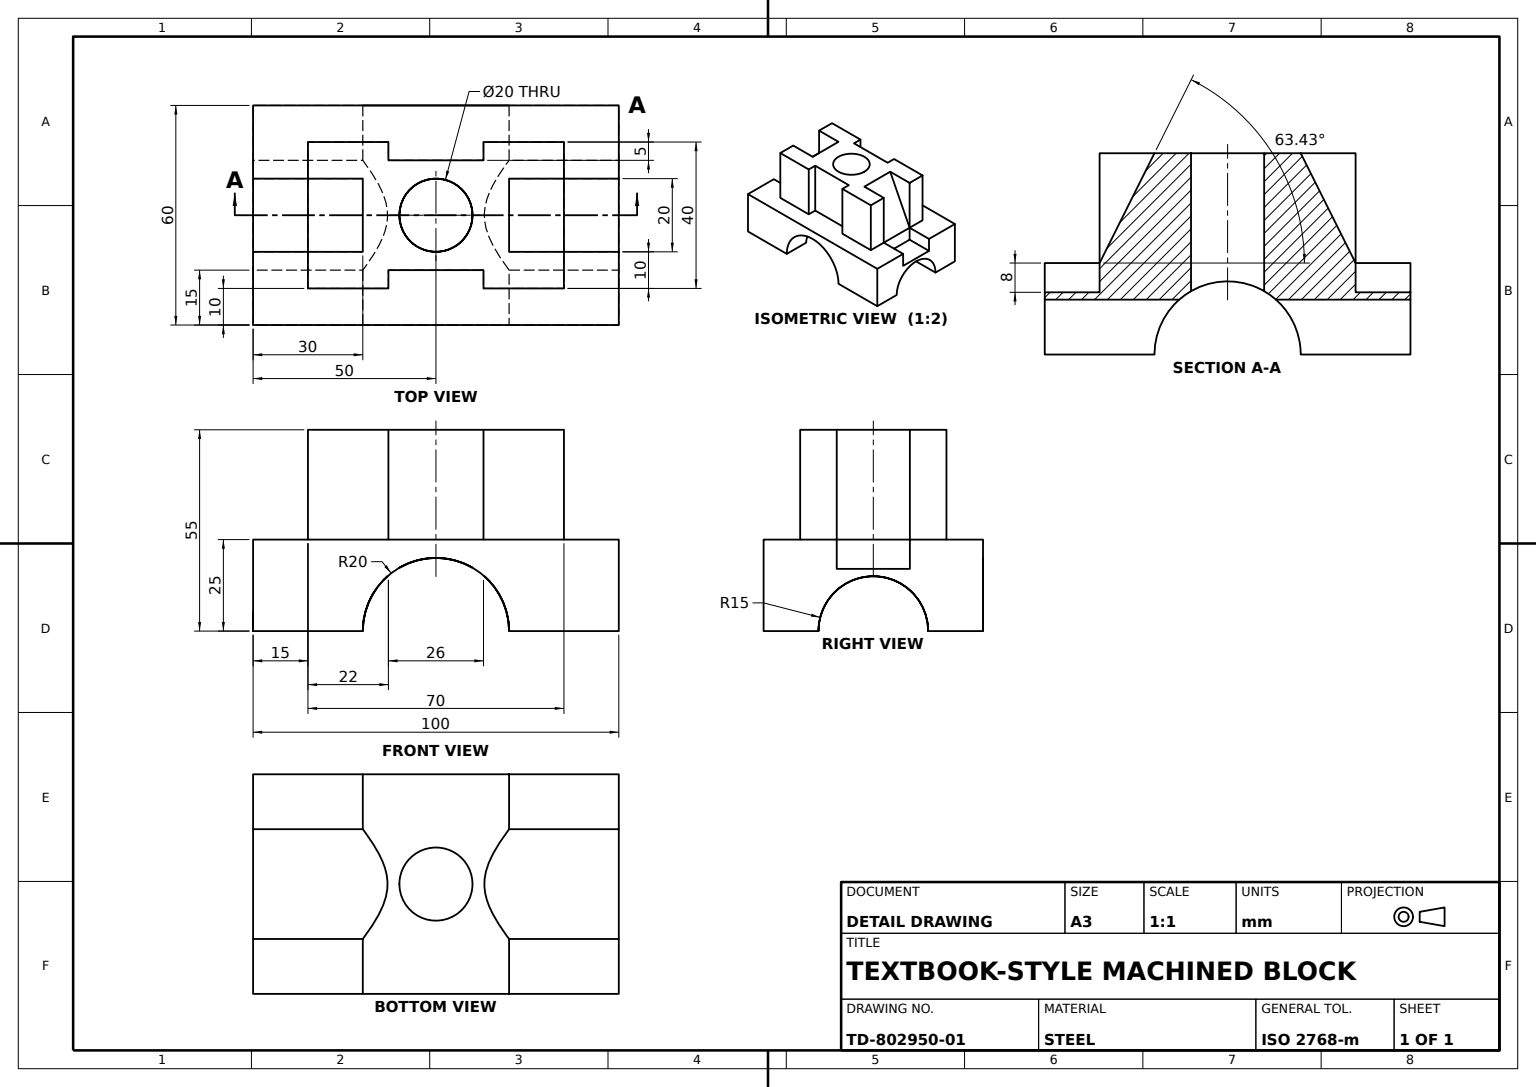
from build123d import *

# Parameters (mm, degrees)
BASE_BLOCK_PROFILE_W        = 100
BASE_BLOCK_PROFILE_H        = 25
BASE_BLOCK_DEPTH            = 30
END_ARCH_CUT_DEPTH          = 106.148704224
END_ARCH_CUT_DEPTH_BACK     = 106.148704224
CENTER_ARCH_CUT_DEPTH       = 80.096460098
UPPER_BLOCK_PROFILE_W       = 40
UPPER_BLOCK_PROFILE_H       = 30
UPPER_BLOCK_DEPTH           = 35
SIDE_SLOT_PROFILE_W         = 5
SIDE_SLOT_PROFILE_H         = 26
SIDE_SLOT_DEPTH             = 30
TOP_BORE_PROFILE_R          = 10
TOP_BORE_20_DEPTH           = 81.156097878
BASE_NOTCH_PROFILE_W        = 20
BASE_NOTCH_PROFILE_H        = 8
BASE_NOTCH_DEPTH            = 15
TRIANGULAR_RELIEF_CUT_DEPTH = 10


with BuildPart() as part:
    # Base Block Profile → Base Block (new, symmetric)
    with BuildSketch(Plane(origin=(0, 0, 0), x_dir=(0, 0, -1), z_dir=(1, 0, 0))):
        Rectangle(BASE_BLOCK_PROFILE_W, BASE_BLOCK_PROFILE_H)
    extrude(amount=BASE_BLOCK_DEPTH, both=True)

    # End Arch Profile → End Arch Cut (cut, two sides: drawn at the far end of the back side and taken through both)
    with BuildSketch(Plane.XY.offset(50).offset(-END_ARCH_CUT_DEPTH_BACK)):
        with BuildLine():
            ThreePointArc((15, -12.5), (0, 2.5), (-15, -12.5))
            Line((-15, -12.5), (15, -12.5))
        make_face()
    extrude(amount=END_ARCH_CUT_DEPTH + END_ARCH_CUT_DEPTH_BACK, mode=Mode.SUBTRACT)

    # Center Arch Profile → Center Arch Cut (cut, through all)
    with BuildSketch(Plane(origin=(30, 0, 0), x_dir=(0, 0, -1), z_dir=(1, 0, 0))):
        with BuildLine():
            ThreePointArc((20, -12.5), (0, 7.5), (-20, -12.5))
            Line((-20, -12.5), (20, -12.5))
        make_face()
    extrude(amount=-CENTER_ARCH_CUT_DEPTH, mode=Mode.SUBTRACT)

    # Upper Block Profile → Upper Block (add, symmetric)
    with BuildSketch(Plane.XY):
        with Locations((0, 27.5)):
            Rectangle(UPPER_BLOCK_PROFILE_W, UPPER_BLOCK_PROFILE_H)
    extrude(amount=UPPER_BLOCK_DEPTH, both=True)

    # Side Slot Profile → Side Slot (cut)
    with BuildSketch(Plane(origin=(0, 42.5, 0), x_dir=(1, 0, 0), z_dir=(0, 1, 0))):
        with Locations((17.5, 0)):
            Rectangle(SIDE_SLOT_PROFILE_W, SIDE_SLOT_PROFILE_H)
    side_slot = extrude(amount=-SIDE_SLOT_DEPTH, mode=Mode.SUBTRACT)

    # Side Slot Mirror: Side Slot across plane
    add(side_slot.mirror(Plane(origin=(0, 0, 0), x_dir=(0, 0, 1), z_dir=(1, 0, 0))), mode=Mode.SUBTRACT)

    # Top Bore Profile → Top Bore Ø20 (cut, through all)
    with BuildSketch(Plane(origin=(0, 42.5, 0), x_dir=(1, 0, 0), z_dir=(0, 1, 0))):
        with Locations(Location((0, 0, 0), (0, 0, 270))):
            Circle(TOP_BORE_PROFILE_R)
    extrude(amount=-TOP_BORE_20_DEPTH, mode=Mode.SUBTRACT)

    # Base Notch Profile → Base Notch (cut)
    with BuildSketch(Plane.XY.offset(50)):
        with Locations((0, 8.5)):
            Rectangle(BASE_NOTCH_PROFILE_W, BASE_NOTCH_PROFILE_H)
    base_notch = extrude(amount=-BASE_NOTCH_DEPTH, mode=Mode.SUBTRACT)

    # Triangular Relief Profile → Triangular Relief Cut (cut, symmetric)
    with BuildSketch(Plane(origin=(0, 0, 0), x_dir=(0, 0, -1), z_dir=(1, 0, 0))):
        Polygon((-35, 12.5), (-20, 42.5), (-35, 42.5), align=None)
    triangular_relief_cut = extrude(amount=TRIANGULAR_RELIEF_CUT_DEPTH, both=True, mode=Mode.SUBTRACT)

    # Notch and Relief Mirror: Base Notch, Triangular Relief Cut across plane
    add(base_notch.mirror(Plane.XY), mode=Mode.SUBTRACT)
    add(triangular_relief_cut.mirror(Plane.XY), mode=Mode.SUBTRACT)


solid = part.part
